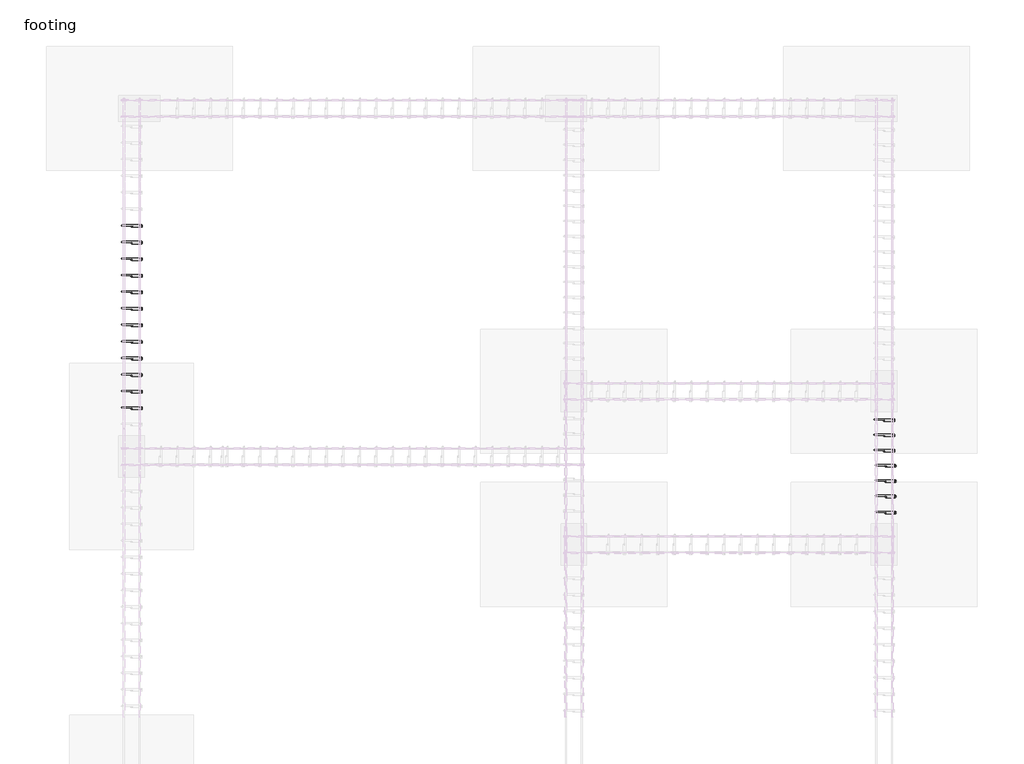
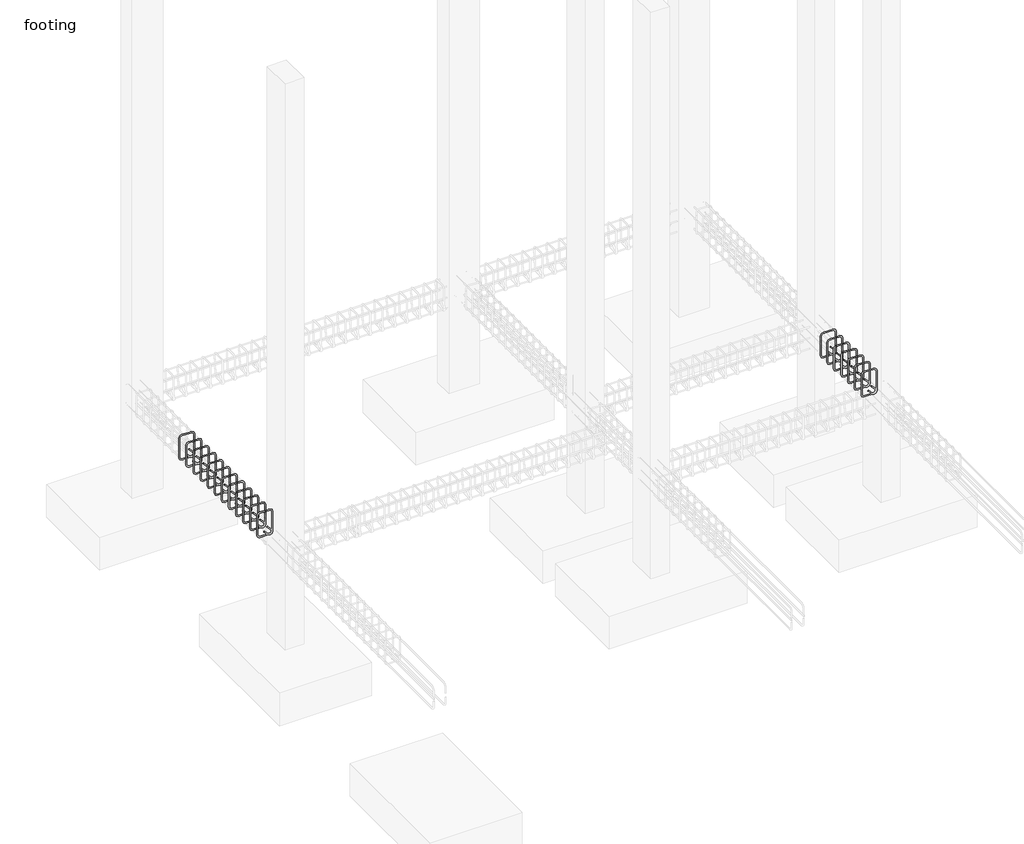
# One storey, part 15 of 21: 19 reinforcing bars.
"""IFC4 building model written with IfcOpenShell, lengths in millimetres."""

from ifc_helpers import new_model, si_unit, point, frame, origin, place, context, project, spatial, polyline, circle_curve, trimmed, segment, composite_curve, element, save
from ifc_brep_helpers import swept_disk

model = new_model("IFC4")

# Units and contexts
model_context = context("Model", 3, world=origin())
ifc_project = project(units=[si_unit("LENGTHUNIT", "METRE", prefix="MILLI")], contexts=[model_context])

# Site, building, storey
site = spatial("IfcSite", under=ifc_project)
building = spatial("IfcBuilding", under=site)
storey = spatial("IfcBuildingStorey", under=building, Name="footing", Elevation=-1524.0)

# Reinforcing bars
placement = place(None, origin())
element("IfcReinforcingBar", 1, at=placement, inside=storey, context=model_context, shape_type="SolidModel", body=[
    swept_disk(composite_curve([segment(polyline([(-12178.1165254, 8042.8456073, -265.9812362), (-12123.251527, 8042.8456073, -320.8462347)]), True, "CONTINUOUS"), segment(trimmed(circle_curve(frame((-12145.7021673, 8042.8456073, -343.296875), z_axis=(0.0, 1.0, 0.0), x_axis=(22.450640299999577, 0.0, 22.450640299999975)), 31.75), [point((-12123.251527, 8042.8456073, -320.8462347))], [point((-12145.7021673, 8042.8456073, -375.046875))], True, "CARTESIAN"), True, "CONTINUOUS"), segment(polyline([(-12145.7021673, 8042.8456073, -375.046875), (-12273.4959173, 8042.8456073, -375.046875)]), True, "CONTINUOUS"), segment(trimmed(circle_curve(frame((-12273.4959173, 8042.8456073, -343.296875), z_axis=(0.0, 1.0, 0.0), x_axis=(0.0, 0.0, -31.75)), 31.75), [point((-12273.4959173, 8042.8456073, -375.046875))], [point((-12305.2459173, 8042.8456073, -343.296875))], True, "CARTESIAN"), True, "CONTINUOUS"), segment(polyline([(-12305.2459173, 8042.8456073, -343.296875), (-12305.2459173, 8042.8456073, -63.103125)]), True, "CONTINUOUS"), segment(trimmed(circle_curve(frame((-12273.565658, 8040.7423536, -63.103125), z_axis=(0.0662442117686417, 0.9978034397651431, 0.0), x_axis=(-31.680259300001126, 2.1032537000000957, 0.0)), 31.75), [point((-12305.2459173, 8042.8456073, -63.103125))], [point((-12273.565658, 8040.7423536, -31.353125))], True, "CARTESIAN"), True, "CONTINUOUS"), segment(polyline([(-12273.565658, 8040.7423536, -31.353125), (-12145.6324265, 8032.248861, -31.353125)]), True, "CONTINUOUS"), segment(trimmed(circle_curve(frame((-12145.6324265, 8032.248861, -63.103125), z_axis=(0.06624421176864169, 0.997803439765143, 0.0), x_axis=(0.0, 0.0, 31.75)), 31.75), [point((-12145.6324265, 8032.248861, -31.353125))], [point((-12113.9521673, 8030.1456073, -63.103125))], True, "CARTESIAN"), True, "CONTINUOUS"), segment(polyline([(-12113.9521673, 8030.1456073, -63.103125), (-12113.9521673, 8030.1456073, -343.296875)]), True, "CONTINUOUS"), segment(trimmed(circle_curve(frame((-12145.7021673, 8030.1456073, -343.296875), z_axis=(0.0, 1.0, 0.0), x_axis=(31.75, 0.0, 0.0)), 31.75), [point((-12113.9521673, 8030.1456073, -343.296875))], [point((-12168.1528076, 8030.1456073, -365.7475153))], True, "CARTESIAN"), True, "CONTINUOUS"), segment(polyline([(-12168.1528076, 8030.1456073, -365.7475153), (-12223.017806, 8030.1456073, -310.8825168)]), True, "CONTINUOUS")], self_intersect=False), 6.35),
])
element("IfcReinforcingBar", 2, at=placement, inside=storey, context=model_context, shape_type="SolidModel", body=[
    swept_disk(composite_curve([segment(polyline([(-12178.1165254, 8205.5456073, -265.9812362), (-12123.251527, 8205.5456073, -320.8462347)]), True, "CONTINUOUS"), segment(trimmed(circle_curve(frame((-12145.7021673, 8205.5456073, -343.296875), z_axis=(0.0, 1.0, 0.0), x_axis=(22.450640299999577, 0.0, 22.450640299999975)), 31.75), [point((-12123.251527, 8205.5456073, -320.8462347))], [point((-12145.7021673, 8205.5456073, -375.046875))], True, "CARTESIAN"), True, "CONTINUOUS"), segment(polyline([(-12145.7021673, 8205.5456073, -375.046875), (-12273.4959173, 8205.5456073, -375.046875)]), True, "CONTINUOUS"), segment(trimmed(circle_curve(frame((-12273.4959173, 8205.5456073, -343.296875), z_axis=(0.0, 1.0, 0.0), x_axis=(0.0, 0.0, -31.75)), 31.75), [point((-12273.4959173, 8205.5456073, -375.046875))], [point((-12305.2459173, 8205.5456073, -343.296875))], True, "CARTESIAN"), True, "CONTINUOUS"), segment(polyline([(-12305.2459173, 8205.5456073, -343.296875), (-12305.2459173, 8205.5456073, -63.103125)]), True, "CONTINUOUS"), segment(trimmed(circle_curve(frame((-12273.565658, 8203.4423536, -63.103125), z_axis=(0.0662442117686417, 0.9978034397651431, 0.0), x_axis=(-31.680259300001126, 2.103253700001005, 0.0)), 31.75), [point((-12305.2459173, 8205.5456073, -63.103125))], [point((-12273.565658, 8203.4423536, -31.353125))], True, "CARTESIAN"), True, "CONTINUOUS"), segment(polyline([(-12273.565658, 8203.4423536, -31.353125), (-12145.6324265, 8194.948861, -31.353125)]), True, "CONTINUOUS"), segment(trimmed(circle_curve(frame((-12145.6324265, 8194.948861, -63.103125), z_axis=(0.06624421176864169, 0.997803439765143, 0.0), x_axis=(0.0, 0.0, 31.75)), 31.75), [point((-12145.6324265, 8194.948861, -31.353125))], [point((-12113.9521673, 8192.8456073, -63.103125))], True, "CARTESIAN"), True, "CONTINUOUS"), segment(polyline([(-12113.9521673, 8192.8456073, -63.103125), (-12113.9521673, 8192.8456073, -343.296875)]), True, "CONTINUOUS"), segment(trimmed(circle_curve(frame((-12145.7021673, 8192.8456073, -343.296875), z_axis=(0.0, 1.0, 0.0), x_axis=(31.75, 0.0, 0.0)), 31.75), [point((-12113.9521673, 8192.8456073, -343.296875))], [point((-12168.1528076, 8192.8456073, -365.7475153))], True, "CARTESIAN"), True, "CONTINUOUS"), segment(polyline([(-12168.1528076, 8192.8456073, -365.7475153), (-12223.017806, 8192.8456073, -310.8825168)]), True, "CONTINUOUS")], self_intersect=False), 6.35),
])
element("IfcReinforcingBar", 3, at=placement, inside=storey, context=model_context, shape_type="SolidModel", body=[
    swept_disk(composite_curve([segment(polyline([(-12178.1165254, 8368.2456073, -265.9812362), (-12123.251527, 8368.2456073, -320.8462347)]), True, "CONTINUOUS"), segment(trimmed(circle_curve(frame((-12145.7021673, 8368.2456073, -343.296875), z_axis=(0.0, 1.0, 0.0), x_axis=(22.450640299999577, 0.0, 22.450640299999975)), 31.75), [point((-12123.251527, 8368.2456073, -320.8462347))], [point((-12145.7021673, 8368.2456073, -375.046875))], True, "CARTESIAN"), True, "CONTINUOUS"), segment(polyline([(-12145.7021673, 8368.2456073, -375.046875), (-12273.4959173, 8368.2456073, -375.046875)]), True, "CONTINUOUS"), segment(trimmed(circle_curve(frame((-12273.4959173, 8368.2456073, -343.296875), z_axis=(0.0, 1.0, 0.0), x_axis=(0.0, 0.0, -31.75)), 31.75), [point((-12273.4959173, 8368.2456073, -375.046875))], [point((-12305.2459173, 8368.2456073, -343.296875))], True, "CARTESIAN"), True, "CONTINUOUS"), segment(polyline([(-12305.2459173, 8368.2456073, -343.296875), (-12305.2459173, 8368.2456073, -63.103125)]), True, "CONTINUOUS"), segment(trimmed(circle_curve(frame((-12273.565658, 8366.1423536, -63.103125), z_axis=(0.0662442117686417, 0.9978034397651431, 0.0), x_axis=(-31.680259300001126, 2.103253699999186, 0.0)), 31.75), [point((-12305.2459173, 8368.2456073, -63.103125))], [point((-12273.565658, 8366.1423536, -31.353125))], True, "CARTESIAN"), True, "CONTINUOUS"), segment(polyline([(-12273.565658, 8366.1423536, -31.353125), (-12145.6324265, 8357.648861, -31.353125)]), True, "CONTINUOUS"), segment(trimmed(circle_curve(frame((-12145.6324265, 8357.648861, -63.103125), z_axis=(0.06624421176864169, 0.997803439765143, 0.0), x_axis=(0.0, 0.0, 31.75)), 31.75), [point((-12145.6324265, 8357.648861, -31.353125))], [point((-12113.9521673, 8355.5456073, -63.103125))], True, "CARTESIAN"), True, "CONTINUOUS"), segment(polyline([(-12113.9521673, 8355.5456073, -63.103125), (-12113.9521673, 8355.5456073, -343.296875)]), True, "CONTINUOUS"), segment(trimmed(circle_curve(frame((-12145.7021673, 8355.5456073, -343.296875), z_axis=(0.0, 1.0, 0.0), x_axis=(31.75, 0.0, 0.0)), 31.75), [point((-12113.9521673, 8355.5456073, -343.296875))], [point((-12168.1528076, 8355.5456073, -365.7475153))], True, "CARTESIAN"), True, "CONTINUOUS"), segment(polyline([(-12168.1528076, 8355.5456073, -365.7475153), (-12223.017806, 8355.5456073, -310.8825168)]), True, "CONTINUOUS")], self_intersect=False), 6.35),
])
element("IfcReinforcingBar", 4, at=placement, inside=storey, context=model_context, shape_type="SolidModel", body=[
    swept_disk(composite_curve([segment(polyline([(-12178.1165254, 8530.9456073, -265.9812362), (-12123.251527, 8530.9456073, -320.8462347)]), True, "CONTINUOUS"), segment(trimmed(circle_curve(frame((-12145.7021673, 8530.9456073, -343.296875), z_axis=(0.0, 1.0, 0.0), x_axis=(22.450640299999577, 0.0, 22.450640299999975)), 31.75), [point((-12123.251527, 8530.9456073, -320.8462347))], [point((-12145.7021673, 8530.9456073, -375.046875))], True, "CARTESIAN"), True, "CONTINUOUS"), segment(polyline([(-12145.7021673, 8530.9456073, -375.046875), (-12273.4959173, 8530.9456073, -375.046875)]), True, "CONTINUOUS"), segment(trimmed(circle_curve(frame((-12273.4959173, 8530.9456073, -343.296875), z_axis=(0.0, 1.0, 0.0), x_axis=(0.0, 0.0, -31.75)), 31.75), [point((-12273.4959173, 8530.9456073, -375.046875))], [point((-12305.2459173, 8530.9456073, -343.296875))], True, "CARTESIAN"), True, "CONTINUOUS"), segment(polyline([(-12305.2459173, 8530.9456073, -343.296875), (-12305.2459173, 8530.9456073, -63.103125)]), True, "CONTINUOUS"), segment(trimmed(circle_curve(frame((-12273.565658, 8528.8423536, -63.103125), z_axis=(0.0662442117686417, 0.9978034397651431, 0.0), x_axis=(-31.680259300001126, 2.103253700001005, 0.0)), 31.75), [point((-12305.2459173, 8530.9456073, -63.103125))], [point((-12273.565658, 8528.8423536, -31.353125))], True, "CARTESIAN"), True, "CONTINUOUS"), segment(polyline([(-12273.565658, 8528.8423536, -31.353125), (-12145.6324265, 8520.348861, -31.353125)]), True, "CONTINUOUS"), segment(trimmed(circle_curve(frame((-12145.6324265, 8520.348861, -63.103125), z_axis=(0.06624421176864169, 0.997803439765143, 0.0), x_axis=(0.0, 0.0, 31.75)), 31.75), [point((-12145.6324265, 8520.348861, -31.353125))], [point((-12113.9521673, 8518.2456073, -63.103125))], True, "CARTESIAN"), True, "CONTINUOUS"), segment(polyline([(-12113.9521673, 8518.2456073, -63.103125), (-12113.9521673, 8518.2456073, -343.296875)]), True, "CONTINUOUS"), segment(trimmed(circle_curve(frame((-12145.7021673, 8518.2456073, -343.296875), z_axis=(0.0, 1.0, 0.0), x_axis=(31.75, 0.0, 0.0)), 31.75), [point((-12113.9521673, 8518.2456073, -343.296875))], [point((-12168.1528076, 8518.2456073, -365.7475153))], True, "CARTESIAN"), True, "CONTINUOUS"), segment(polyline([(-12168.1528076, 8518.2456073, -365.7475153), (-12223.017806, 8518.2456073, -310.8825168)]), True, "CONTINUOUS")], self_intersect=False), 6.35),
])
element("IfcReinforcingBar", 5, at=placement, inside=storey, context=model_context, shape_type="SolidModel", body=[
    swept_disk(composite_curve([segment(polyline([(-12178.1165254, 8693.6456073, -265.9812362), (-12123.251527, 8693.6456073, -320.8462347)]), True, "CONTINUOUS"), segment(trimmed(circle_curve(frame((-12145.7021673, 8693.6456073, -343.296875), z_axis=(0.0, 1.0, 0.0), x_axis=(22.450640299999577, 0.0, 22.450640299999975)), 31.75), [point((-12123.251527, 8693.6456073, -320.8462347))], [point((-12145.7021673, 8693.6456073, -375.046875))], True, "CARTESIAN"), True, "CONTINUOUS"), segment(polyline([(-12145.7021673, 8693.6456073, -375.046875), (-12273.4959173, 8693.6456073, -375.046875)]), True, "CONTINUOUS"), segment(trimmed(circle_curve(frame((-12273.4959173, 8693.6456073, -343.296875), z_axis=(0.0, 1.0, 0.0), x_axis=(0.0, 0.0, -31.75)), 31.75), [point((-12273.4959173, 8693.6456073, -375.046875))], [point((-12305.2459173, 8693.6456073, -343.296875))], True, "CARTESIAN"), True, "CONTINUOUS"), segment(polyline([(-12305.2459173, 8693.6456073, -343.296875), (-12305.2459173, 8693.6456073, -63.103125)]), True, "CONTINUOUS"), segment(trimmed(circle_curve(frame((-12273.565658, 8691.5423536, -63.103125), z_axis=(0.0662442117686417, 0.9978034397651431, 0.0), x_axis=(-31.680259300001126, 2.103253700001005, 0.0)), 31.75), [point((-12305.2459173, 8693.6456073, -63.103125))], [point((-12273.565658, 8691.5423536, -31.353125))], True, "CARTESIAN"), True, "CONTINUOUS"), segment(polyline([(-12273.565658, 8691.5423536, -31.353125), (-12145.6324265, 8683.048861, -31.353125)]), True, "CONTINUOUS"), segment(trimmed(circle_curve(frame((-12145.6324265, 8683.048861, -63.103125), z_axis=(0.06624421176864169, 0.997803439765143, 0.0), x_axis=(0.0, 0.0, 31.75)), 31.75), [point((-12145.6324265, 8683.048861, -31.353125))], [point((-12113.9521673, 8680.9456073, -63.103125))], True, "CARTESIAN"), True, "CONTINUOUS"), segment(polyline([(-12113.9521673, 8680.9456073, -63.103125), (-12113.9521673, 8680.9456073, -343.296875)]), True, "CONTINUOUS"), segment(trimmed(circle_curve(frame((-12145.7021673, 8680.9456073, -343.296875), z_axis=(0.0, 1.0, 0.0), x_axis=(31.75, 0.0, 0.0)), 31.75), [point((-12113.9521673, 8680.9456073, -343.296875))], [point((-12168.1528076, 8680.9456073, -365.7475153))], True, "CARTESIAN"), True, "CONTINUOUS"), segment(polyline([(-12168.1528076, 8680.9456073, -365.7475153), (-12223.017806, 8680.9456073, -310.8825168)]), True, "CONTINUOUS")], self_intersect=False), 6.35),
])
element("IfcReinforcingBar", 6, at=placement, inside=storey, context=model_context, shape_type="SolidModel", body=[
    swept_disk(composite_curve([segment(polyline([(-12178.1165254, 8856.3456073, -265.9812362), (-12123.251527, 8856.3456073, -320.8462347)]), True, "CONTINUOUS"), segment(trimmed(circle_curve(frame((-12145.7021673, 8856.3456073, -343.296875), z_axis=(0.0, 1.0, 0.0), x_axis=(22.450640299999577, 0.0, 22.450640299999975)), 31.75), [point((-12123.251527, 8856.3456073, -320.8462347))], [point((-12145.7021673, 8856.3456073, -375.046875))], True, "CARTESIAN"), True, "CONTINUOUS"), segment(polyline([(-12145.7021673, 8856.3456073, -375.046875), (-12273.4959173, 8856.3456073, -375.046875)]), True, "CONTINUOUS"), segment(trimmed(circle_curve(frame((-12273.4959173, 8856.3456073, -343.296875), z_axis=(0.0, 1.0, 0.0), x_axis=(0.0, 0.0, -31.75)), 31.75), [point((-12273.4959173, 8856.3456073, -375.046875))], [point((-12305.2459173, 8856.3456073, -343.296875))], True, "CARTESIAN"), True, "CONTINUOUS"), segment(polyline([(-12305.2459173, 8856.3456073, -343.296875), (-12305.2459173, 8856.3456073, -63.103125)]), True, "CONTINUOUS"), segment(trimmed(circle_curve(frame((-12273.565658, 8854.2423536, -63.103125), z_axis=(0.0662442117686417, 0.9978034397651431, 0.0), x_axis=(-31.680259300001126, 2.103253699999186, 0.0)), 31.75), [point((-12305.2459173, 8856.3456073, -63.103125))], [point((-12273.565658, 8854.2423536, -31.353125))], True, "CARTESIAN"), True, "CONTINUOUS"), segment(polyline([(-12273.565658, 8854.2423536, -31.353125), (-12145.6324265, 8845.748861, -31.353125)]), True, "CONTINUOUS"), segment(trimmed(circle_curve(frame((-12145.6324265, 8845.748861, -63.103125), z_axis=(0.06624421176864169, 0.997803439765143, 0.0), x_axis=(0.0, 0.0, 31.75)), 31.75), [point((-12145.6324265, 8845.748861, -31.353125))], [point((-12113.9521673, 8843.6456073, -63.103125))], True, "CARTESIAN"), True, "CONTINUOUS"), segment(polyline([(-12113.9521673, 8843.6456073, -63.103125), (-12113.9521673, 8843.6456073, -343.296875)]), True, "CONTINUOUS"), segment(trimmed(circle_curve(frame((-12145.7021673, 8843.6456073, -343.296875), z_axis=(0.0, 1.0, 0.0), x_axis=(31.75, 0.0, 0.0)), 31.75), [point((-12113.9521673, 8843.6456073, -343.296875))], [point((-12168.1528076, 8843.6456073, -365.7475153))], True, "CARTESIAN"), True, "CONTINUOUS"), segment(polyline([(-12168.1528076, 8843.6456073, -365.7475153), (-12223.017806, 8843.6456073, -310.8825168)]), True, "CONTINUOUS")], self_intersect=False), 6.35),
])
element("IfcReinforcingBar", 7, at=placement, inside=storey, context=model_context, shape_type="SolidModel", body=[
    swept_disk(composite_curve([segment(polyline([(-12178.1165254, 9019.0456073, -265.9812362), (-12123.251527, 9019.0456073, -320.8462347)]), True, "CONTINUOUS"), segment(trimmed(circle_curve(frame((-12145.7021673, 9019.0456073, -343.296875), z_axis=(0.0, 1.0, 0.0), x_axis=(22.450640299999577, 0.0, 22.450640299999975)), 31.75), [point((-12123.251527, 9019.0456073, -320.8462347))], [point((-12145.7021673, 9019.0456073, -375.046875))], True, "CARTESIAN"), True, "CONTINUOUS"), segment(polyline([(-12145.7021673, 9019.0456073, -375.046875), (-12273.4959173, 9019.0456073, -375.046875)]), True, "CONTINUOUS"), segment(trimmed(circle_curve(frame((-12273.4959173, 9019.0456073, -343.296875), z_axis=(0.0, 1.0, 0.0), x_axis=(0.0, 0.0, -31.75)), 31.75), [point((-12273.4959173, 9019.0456073, -375.046875))], [point((-12305.2459173, 9019.0456073, -343.296875))], True, "CARTESIAN"), True, "CONTINUOUS"), segment(polyline([(-12305.2459173, 9019.0456073, -343.296875), (-12305.2459173, 9019.0456073, -63.103125)]), True, "CONTINUOUS"), segment(trimmed(circle_curve(frame((-12273.565658, 9016.9423536, -63.103125), z_axis=(0.0662442117686417, 0.9978034397651431, 0.0), x_axis=(-31.680259300001126, 2.103253700001005, 0.0)), 31.75), [point((-12305.2459173, 9019.0456073, -63.103125))], [point((-12273.565658, 9016.9423536, -31.353125))], True, "CARTESIAN"), True, "CONTINUOUS"), segment(polyline([(-12273.565658, 9016.9423536, -31.353125), (-12145.6324265, 9008.448861, -31.353125)]), True, "CONTINUOUS"), segment(trimmed(circle_curve(frame((-12145.6324265, 9008.448861, -63.103125), z_axis=(0.06624421176864169, 0.997803439765143, 0.0), x_axis=(0.0, 0.0, 31.75)), 31.75), [point((-12145.6324265, 9008.448861, -31.353125))], [point((-12113.9521673, 9006.3456073, -63.103125))], True, "CARTESIAN"), True, "CONTINUOUS"), segment(polyline([(-12113.9521673, 9006.3456073, -63.103125), (-12113.9521673, 9006.3456073, -343.296875)]), True, "CONTINUOUS"), segment(trimmed(circle_curve(frame((-12145.7021673, 9006.3456073, -343.296875), z_axis=(0.0, 1.0, 0.0), x_axis=(31.75, 0.0, 0.0)), 31.75), [point((-12113.9521673, 9006.3456073, -343.296875))], [point((-12168.1528076, 9006.3456073, -365.7475153))], True, "CARTESIAN"), True, "CONTINUOUS"), segment(polyline([(-12168.1528076, 9006.3456073, -365.7475153), (-12223.017806, 9006.3456073, -310.8825168)]), True, "CONTINUOUS")], self_intersect=False), 6.35),
])
element("IfcReinforcingBar", 8, at=placement, inside=storey, context=model_context, shape_type="SolidModel", body=[
    swept_disk(composite_curve([segment(polyline([(-12178.1165254, 9181.7456073, -265.9812362), (-12123.251527, 9181.7456073, -320.8462347)]), True, "CONTINUOUS"), segment(trimmed(circle_curve(frame((-12145.7021673, 9181.7456073, -343.296875), z_axis=(0.0, 1.0, 0.0), x_axis=(22.450640299999577, 0.0, 22.450640299999975)), 31.75), [point((-12123.251527, 9181.7456073, -320.8462347))], [point((-12145.7021673, 9181.7456073, -375.046875))], True, "CARTESIAN"), True, "CONTINUOUS"), segment(polyline([(-12145.7021673, 9181.7456073, -375.046875), (-12273.4959173, 9181.7456073, -375.046875)]), True, "CONTINUOUS"), segment(trimmed(circle_curve(frame((-12273.4959173, 9181.7456073, -343.296875), z_axis=(0.0, 1.0, 0.0), x_axis=(0.0, 0.0, -31.75)), 31.75), [point((-12273.4959173, 9181.7456073, -375.046875))], [point((-12305.2459173, 9181.7456073, -343.296875))], True, "CARTESIAN"), True, "CONTINUOUS"), segment(polyline([(-12305.2459173, 9181.7456073, -343.296875), (-12305.2459173, 9181.7456073, -63.103125)]), True, "CONTINUOUS"), segment(trimmed(circle_curve(frame((-12273.565658, 9179.6423536, -63.103125), z_axis=(0.0662442117686417, 0.9978034397651431, 0.0), x_axis=(-31.680259300001126, 2.103253699999186, 0.0)), 31.75), [point((-12305.2459173, 9181.7456073, -63.103125))], [point((-12273.565658, 9179.6423536, -31.353125))], True, "CARTESIAN"), True, "CONTINUOUS"), segment(polyline([(-12273.565658, 9179.6423536, -31.353125), (-12145.6324265, 9171.148861, -31.353125)]), True, "CONTINUOUS"), segment(trimmed(circle_curve(frame((-12145.6324265, 9171.148861, -63.103125), z_axis=(0.06624421176864169, 0.997803439765143, 0.0), x_axis=(0.0, 0.0, 31.75)), 31.75), [point((-12145.6324265, 9171.148861, -31.353125))], [point((-12113.9521673, 9169.0456073, -63.103125))], True, "CARTESIAN"), True, "CONTINUOUS"), segment(polyline([(-12113.9521673, 9169.0456073, -63.103125), (-12113.9521673, 9169.0456073, -343.296875)]), True, "CONTINUOUS"), segment(trimmed(circle_curve(frame((-12145.7021673, 9169.0456073, -343.296875), z_axis=(0.0, 1.0, 0.0), x_axis=(31.75, 0.0, 0.0)), 31.75), [point((-12113.9521673, 9169.0456073, -343.296875))], [point((-12168.1528076, 9169.0456073, -365.7475153))], True, "CARTESIAN"), True, "CONTINUOUS"), segment(polyline([(-12168.1528076, 9169.0456073, -365.7475153), (-12223.017806, 9169.0456073, -310.8825168)]), True, "CONTINUOUS")], self_intersect=False), 6.35),
])
element("IfcReinforcingBar", 9, at=placement, inside=storey, context=model_context, shape_type="SolidModel", body=[
    swept_disk(composite_curve([segment(polyline([(-12178.1165254, 9344.4456073, -265.9812362), (-12123.251527, 9344.4456073, -320.8462347)]), True, "CONTINUOUS"), segment(trimmed(circle_curve(frame((-12145.7021673, 9344.4456073, -343.296875), z_axis=(0.0, 1.0, 0.0), x_axis=(22.450640299999577, 0.0, 22.450640299999975)), 31.75), [point((-12123.251527, 9344.4456073, -320.8462347))], [point((-12145.7021673, 9344.4456073, -375.046875))], True, "CARTESIAN"), True, "CONTINUOUS"), segment(polyline([(-12145.7021673, 9344.4456073, -375.046875), (-12273.4959173, 9344.4456073, -375.046875)]), True, "CONTINUOUS"), segment(trimmed(circle_curve(frame((-12273.4959173, 9344.4456073, -343.296875), z_axis=(0.0, 1.0, 0.0), x_axis=(0.0, 0.0, -31.75)), 31.75), [point((-12273.4959173, 9344.4456073, -375.046875))], [point((-12305.2459173, 9344.4456073, -343.296875))], True, "CARTESIAN"), True, "CONTINUOUS"), segment(polyline([(-12305.2459173, 9344.4456073, -343.296875), (-12305.2459173, 9344.4456073, -63.103125)]), True, "CONTINUOUS"), segment(trimmed(circle_curve(frame((-12273.565658, 9342.3423536, -63.103125), z_axis=(0.0662442117686417, 0.9978034397651431, 0.0), x_axis=(-31.680259300001126, 2.103253700001005, 0.0)), 31.75), [point((-12305.2459173, 9344.4456073, -63.103125))], [point((-12273.565658, 9342.3423536, -31.353125))], True, "CARTESIAN"), True, "CONTINUOUS"), segment(polyline([(-12273.565658, 9342.3423536, -31.353125), (-12145.6324265, 9333.848861, -31.353125)]), True, "CONTINUOUS"), segment(trimmed(circle_curve(frame((-12145.6324265, 9333.848861, -63.103125), z_axis=(0.06624421176864169, 0.997803439765143, 0.0), x_axis=(0.0, 0.0, 31.75)), 31.75), [point((-12145.6324265, 9333.848861, -31.353125))], [point((-12113.9521673, 9331.7456073, -63.103125))], True, "CARTESIAN"), True, "CONTINUOUS"), segment(polyline([(-12113.9521673, 9331.7456073, -63.103125), (-12113.9521673, 9331.7456073, -343.296875)]), True, "CONTINUOUS"), segment(trimmed(circle_curve(frame((-12145.7021673, 9331.7456073, -343.296875), z_axis=(0.0, 1.0, 0.0), x_axis=(31.75, 0.0, 0.0)), 31.75), [point((-12113.9521673, 9331.7456073, -343.296875))], [point((-12168.1528076, 9331.7456073, -365.7475153))], True, "CARTESIAN"), True, "CONTINUOUS"), segment(polyline([(-12168.1528076, 9331.7456073, -365.7475153), (-12223.017806, 9331.7456073, -310.8825168)]), True, "CONTINUOUS")], self_intersect=False), 6.35),
])
element("IfcReinforcingBar", 10, at=placement, inside=storey, context=model_context, shape_type="SolidModel", body=[
    swept_disk(composite_curve([segment(polyline([(-12178.1165254, 9507.1456073, -265.9812362), (-12123.251527, 9507.1456073, -320.8462347)]), True, "CONTINUOUS"), segment(trimmed(circle_curve(frame((-12145.7021673, 9507.1456073, -343.296875), z_axis=(0.0, 1.0, 0.0), x_axis=(22.450640299999577, 0.0, 22.450640299999975)), 31.75), [point((-12123.251527, 9507.1456073, -320.8462347))], [point((-12145.7021673, 9507.1456073, -375.046875))], True, "CARTESIAN"), True, "CONTINUOUS"), segment(polyline([(-12145.7021673, 9507.1456073, -375.046875), (-12273.4959173, 9507.1456073, -375.046875)]), True, "CONTINUOUS"), segment(trimmed(circle_curve(frame((-12273.4959173, 9507.1456073, -343.296875), z_axis=(0.0, 1.0, 0.0), x_axis=(0.0, 0.0, -31.75)), 31.75), [point((-12273.4959173, 9507.1456073, -375.046875))], [point((-12305.2459173, 9507.1456073, -343.296875))], True, "CARTESIAN"), True, "CONTINUOUS"), segment(polyline([(-12305.2459173, 9507.1456073, -343.296875), (-12305.2459173, 9507.1456073, -63.103125)]), True, "CONTINUOUS"), segment(trimmed(circle_curve(frame((-12273.565658, 9505.0423536, -63.103125), z_axis=(0.0662442117686417, 0.9978034397651431, 0.0), x_axis=(-31.680259300001126, 2.103253700001005, 0.0)), 31.75), [point((-12305.2459173, 9507.1456073, -63.103125))], [point((-12273.565658, 9505.0423536, -31.353125))], True, "CARTESIAN"), True, "CONTINUOUS"), segment(polyline([(-12273.565658, 9505.0423536, -31.353125), (-12145.6324265, 9496.548861, -31.353125)]), True, "CONTINUOUS"), segment(trimmed(circle_curve(frame((-12145.6324265, 9496.548861, -63.103125), z_axis=(0.06624421176864169, 0.997803439765143, 0.0), x_axis=(0.0, 0.0, 31.75)), 31.75), [point((-12145.6324265, 9496.548861, -31.353125))], [point((-12113.9521673, 9494.4456073, -63.103125))], True, "CARTESIAN"), True, "CONTINUOUS"), segment(polyline([(-12113.9521673, 9494.4456073, -63.103125), (-12113.9521673, 9494.4456073, -343.296875)]), True, "CONTINUOUS"), segment(trimmed(circle_curve(frame((-12145.7021673, 9494.4456073, -343.296875), z_axis=(0.0, 1.0, 0.0), x_axis=(31.75, 0.0, 0.0)), 31.75), [point((-12113.9521673, 9494.4456073, -343.296875))], [point((-12168.1528076, 9494.4456073, -365.7475153))], True, "CARTESIAN"), True, "CONTINUOUS"), segment(polyline([(-12168.1528076, 9494.4456073, -365.7475153), (-12223.017806, 9494.4456073, -310.8825168)]), True, "CONTINUOUS")], self_intersect=False), 6.35),
])
element("IfcReinforcingBar", 11, at=placement, inside=storey, context=model_context, shape_type="SolidModel", body=[
    swept_disk(composite_curve([segment(polyline([(-12178.1165254, 9669.8456073, -265.9812362), (-12123.251527, 9669.8456073, -320.8462347)]), True, "CONTINUOUS"), segment(trimmed(circle_curve(frame((-12145.7021673, 9669.8456073, -343.296875), z_axis=(0.0, 1.0, 0.0), x_axis=(22.450640299999577, 0.0, 22.450640299999975)), 31.75), [point((-12123.251527, 9669.8456073, -320.8462347))], [point((-12145.7021673, 9669.8456073, -375.046875))], True, "CARTESIAN"), True, "CONTINUOUS"), segment(polyline([(-12145.7021673, 9669.8456073, -375.046875), (-12273.4959173, 9669.8456073, -375.046875)]), True, "CONTINUOUS"), segment(trimmed(circle_curve(frame((-12273.4959173, 9669.8456073, -343.296875), z_axis=(0.0, 1.0, 0.0), x_axis=(0.0, 0.0, -31.75)), 31.75), [point((-12273.4959173, 9669.8456073, -375.046875))], [point((-12305.2459173, 9669.8456073, -343.296875))], True, "CARTESIAN"), True, "CONTINUOUS"), segment(polyline([(-12305.2459173, 9669.8456073, -343.296875), (-12305.2459173, 9669.8456073, -63.103125)]), True, "CONTINUOUS"), segment(trimmed(circle_curve(frame((-12273.565658, 9667.7423536, -63.103125), z_axis=(0.0662442117686417, 0.9978034397651431, 0.0), x_axis=(-31.680259300001126, 2.103253699999186, 0.0)), 31.75), [point((-12305.2459173, 9669.8456073, -63.103125))], [point((-12273.565658, 9667.7423536, -31.353125))], True, "CARTESIAN"), True, "CONTINUOUS"), segment(polyline([(-12273.565658, 9667.7423536, -31.353125), (-12145.6324265, 9659.248861, -31.353125)]), True, "CONTINUOUS"), segment(trimmed(circle_curve(frame((-12145.6324265, 9659.248861, -63.103125), z_axis=(0.06624421176864169, 0.997803439765143, 0.0), x_axis=(0.0, 0.0, 31.75)), 31.75), [point((-12145.6324265, 9659.248861, -31.353125))], [point((-12113.9521673, 9657.1456073, -63.103125))], True, "CARTESIAN"), True, "CONTINUOUS"), segment(polyline([(-12113.9521673, 9657.1456073, -63.103125), (-12113.9521673, 9657.1456073, -343.296875)]), True, "CONTINUOUS"), segment(trimmed(circle_curve(frame((-12145.7021673, 9657.1456073, -343.296875), z_axis=(0.0, 1.0, 0.0), x_axis=(31.75, 0.0, 0.0)), 31.75), [point((-12113.9521673, 9657.1456073, -343.296875))], [point((-12168.1528076, 9657.1456073, -365.7475153))], True, "CARTESIAN"), True, "CONTINUOUS"), segment(polyline([(-12168.1528076, 9657.1456073, -365.7475153), (-12223.017806, 9657.1456073, -310.8825168)]), True, "CONTINUOUS")], self_intersect=False), 6.35),
])
element("IfcReinforcingBar", 12, at=placement, inside=storey, context=model_context, shape_type="SolidModel", body=[
    swept_disk(composite_curve([segment(polyline([(-12178.1165254, 9832.5456073, -265.9812362), (-12123.251527, 9832.5456073, -320.8462347)]), True, "CONTINUOUS"), segment(trimmed(circle_curve(frame((-12145.7021673, 9832.5456073, -343.296875), z_axis=(0.0, 1.0, 0.0), x_axis=(22.450640299999577, 0.0, 22.450640299999975)), 31.75), [point((-12123.251527, 9832.5456073, -320.8462347))], [point((-12145.7021673, 9832.5456073, -375.046875))], True, "CARTESIAN"), True, "CONTINUOUS"), segment(polyline([(-12145.7021673, 9832.5456073, -375.046875), (-12273.4959173, 9832.5456073, -375.046875)]), True, "CONTINUOUS"), segment(trimmed(circle_curve(frame((-12273.4959173, 9832.5456073, -343.296875), z_axis=(0.0, 1.0, 0.0), x_axis=(0.0, 0.0, -31.75)), 31.75), [point((-12273.4959173, 9832.5456073, -375.046875))], [point((-12305.2459173, 9832.5456073, -343.296875))], True, "CARTESIAN"), True, "CONTINUOUS"), segment(polyline([(-12305.2459173, 9832.5456073, -343.296875), (-12305.2459173, 9832.5456073, -63.103125)]), True, "CONTINUOUS"), segment(trimmed(circle_curve(frame((-12273.565658, 9830.4423536, -63.103125), z_axis=(0.0662442117686417, 0.9978034397651431, 0.0), x_axis=(-31.680259300001126, 2.103253700001005, 0.0)), 31.75), [point((-12305.2459173, 9832.5456073, -63.103125))], [point((-12273.565658, 9830.4423536, -31.353125))], True, "CARTESIAN"), True, "CONTINUOUS"), segment(polyline([(-12273.565658, 9830.4423536, -31.353125), (-12145.6324265, 9821.948861, -31.353125)]), True, "CONTINUOUS"), segment(trimmed(circle_curve(frame((-12145.6324265, 9821.948861, -63.103125), z_axis=(0.06624421176864169, 0.997803439765143, 0.0), x_axis=(0.0, 0.0, 31.75)), 31.75), [point((-12145.6324265, 9821.948861, -31.353125))], [point((-12113.9521673, 9819.8456073, -63.103125))], True, "CARTESIAN"), True, "CONTINUOUS"), segment(polyline([(-12113.9521673, 9819.8456073, -63.103125), (-12113.9521673, 9819.8456073, -343.296875)]), True, "CONTINUOUS"), segment(trimmed(circle_curve(frame((-12145.7021673, 9819.8456073, -343.296875), z_axis=(0.0, 1.0, 0.0), x_axis=(31.75, 0.0, 0.0)), 31.75), [point((-12113.9521673, 9819.8456073, -343.296875))], [point((-12168.1528076, 9819.8456073, -365.7475153))], True, "CARTESIAN"), True, "CONTINUOUS"), segment(polyline([(-12168.1528076, 9819.8456073, -365.7475153), (-12223.017806, 9819.8456073, -310.8825168)]), True, "CONTINUOUS")], self_intersect=False), 6.35),
])
element("IfcReinforcingBar", 13, at=placement, inside=storey, context=model_context, shape_type="SolidModel", body=[
    swept_disk(composite_curve([segment(polyline([(-4786.7165254, 7925.2699494, -265.9812362), (-4731.851527, 7925.2699494, -320.8462347)]), True, "CONTINUOUS"), segment(trimmed(circle_curve(frame((-4754.3021673, 7925.2699494, -343.296875), z_axis=(0.0, 1.0, 0.0), x_axis=(22.450640300000487, 0.0, 22.450640299999975)), 31.75), [point((-4731.851527, 7925.2699494, -320.8462347))], [point((-4754.3021673, 7925.2699494, -375.046875))], True, "CARTESIAN"), True, "CONTINUOUS"), segment(polyline([(-4754.3021673, 7925.2699494, -375.046875), (-4882.0959173, 7925.2699494, -375.046875)]), True, "CONTINUOUS"), segment(trimmed(circle_curve(frame((-4882.0959173, 7925.2699494, -343.296875), z_axis=(0.0, 1.0, 0.0), x_axis=(0.0, 0.0, -31.75)), 31.75), [point((-4882.0959173, 7925.2699494, -375.046875))], [point((-4913.8459173, 7925.2699494, -343.296875))], True, "CARTESIAN"), True, "CONTINUOUS"), segment(polyline([(-4913.8459173, 7925.2699494, -343.296875), (-4913.8459173, 7925.2699494, -63.103125)]), True, "CONTINUOUS"), segment(trimmed(circle_curve(frame((-4882.165658, 7923.1666957, -63.103125), z_axis=(0.06624421176864137, 0.9978034397651431, 0.0), x_axis=(-31.680259300000216, 2.1032537000000957, 0.0)), 31.75), [point((-4913.8459173, 7925.2699494, -63.103125))], [point((-4882.165658, 7923.1666957, -31.353125))], True, "CARTESIAN"), True, "CONTINUOUS"), segment(polyline([(-4882.165658, 7923.1666957, -31.353125), (-4754.2324265, 7914.6732031, -31.353125)]), True, "CONTINUOUS"), segment(trimmed(circle_curve(frame((-4754.2324265, 7914.6732031, -63.103125), z_axis=(0.06624421176864137, 0.9978034397651431, 0.0), x_axis=(0.0, 0.0, 31.75)), 31.75), [point((-4754.2324265, 7914.6732031, -31.353125))], [point((-4722.5521673, 7912.5699494, -63.103125))], True, "CARTESIAN"), True, "CONTINUOUS"), segment(polyline([(-4722.5521673, 7912.5699494, -63.103125), (-4722.5521673, 7912.5699494, -343.296875)]), True, "CONTINUOUS"), segment(trimmed(circle_curve(frame((-4754.3021673, 7912.5699494, -343.296875), z_axis=(0.0, 1.0, 0.0), x_axis=(31.75, 0.0, 0.0)), 31.75), [point((-4722.5521673, 7912.5699494, -343.296875))], [point((-4776.7528076, 7912.5699494, -365.7475153))], True, "CARTESIAN"), True, "CONTINUOUS"), segment(polyline([(-4776.7528076, 7912.5699494, -365.7475153), (-4831.617806, 7912.5699494, -310.8825168)]), True, "CONTINUOUS")], self_intersect=False), 6.35),
])
element("IfcReinforcingBar", 14, at=placement, inside=storey, context=model_context, shape_type="SolidModel", body=[
    swept_disk(composite_curve([segment(polyline([(-4786.7165254, 7775.2699494, -265.9812362), (-4731.851527, 7775.2699494, -320.8462347)]), True, "CONTINUOUS"), segment(trimmed(circle_curve(frame((-4754.3021673, 7775.2699494, -343.296875), z_axis=(0.0, 1.0, 0.0), x_axis=(22.450640300000487, 0.0, 22.450640299999975)), 31.75), [point((-4731.851527, 7775.2699494, -320.8462347))], [point((-4754.3021673, 7775.2699494, -375.046875))], True, "CARTESIAN"), True, "CONTINUOUS"), segment(polyline([(-4754.3021673, 7775.2699494, -375.046875), (-4882.0959173, 7775.2699494, -375.046875)]), True, "CONTINUOUS"), segment(trimmed(circle_curve(frame((-4882.0959173, 7775.2699494, -343.296875), z_axis=(0.0, 1.0, 0.0), x_axis=(0.0, 0.0, -31.75)), 31.75), [point((-4882.0959173, 7775.2699494, -375.046875))], [point((-4913.8459173, 7775.2699494, -343.296875))], True, "CARTESIAN"), True, "CONTINUOUS"), segment(polyline([(-4913.8459173, 7775.2699494, -343.296875), (-4913.8459173, 7775.2699494, -63.103125)]), True, "CONTINUOUS"), segment(trimmed(circle_curve(frame((-4882.165658, 7773.1666957, -63.103125), z_axis=(0.06624421176864137, 0.9978034397651431, 0.0), x_axis=(-31.680259300000216, 2.1032537000000957, 0.0)), 31.75), [point((-4913.8459173, 7775.2699494, -63.103125))], [point((-4882.165658, 7773.1666957, -31.353125))], True, "CARTESIAN"), True, "CONTINUOUS"), segment(polyline([(-4882.165658, 7773.1666957, -31.353125), (-4754.2324265, 7764.6732031, -31.353125)]), True, "CONTINUOUS"), segment(trimmed(circle_curve(frame((-4754.2324265, 7764.6732031, -63.103125), z_axis=(0.06624421176864137, 0.9978034397651431, 0.0), x_axis=(0.0, 0.0, 31.75)), 31.75), [point((-4754.2324265, 7764.6732031, -31.353125))], [point((-4722.5521673, 7762.5699494, -63.103125))], True, "CARTESIAN"), True, "CONTINUOUS"), segment(polyline([(-4722.5521673, 7762.5699494, -63.103125), (-4722.5521673, 7762.5699494, -343.296875)]), True, "CONTINUOUS"), segment(trimmed(circle_curve(frame((-4754.3021673, 7762.5699494, -343.296875), z_axis=(0.0, 1.0, 0.0), x_axis=(31.75, 0.0, 0.0)), 31.75), [point((-4722.5521673, 7762.5699494, -343.296875))], [point((-4776.7528076, 7762.5699494, -365.7475153))], True, "CARTESIAN"), True, "CONTINUOUS"), segment(polyline([(-4776.7528076, 7762.5699494, -365.7475153), (-4831.617806, 7762.5699494, -310.8825168)]), True, "CONTINUOUS")], self_intersect=False), 6.35),
])
element("IfcReinforcingBar", 15, at=placement, inside=storey, context=model_context, shape_type="SolidModel", body=[
    swept_disk(composite_curve([segment(polyline([(-4786.7165254, 7625.2699494, -265.9812362), (-4731.851527, 7625.2699494, -320.8462347)]), True, "CONTINUOUS"), segment(trimmed(circle_curve(frame((-4754.3021673, 7625.2699494, -343.296875), z_axis=(0.0, 1.0, 0.0), x_axis=(22.450640300000487, 0.0, 22.450640299999975)), 31.75), [point((-4731.851527, 7625.2699494, -320.8462347))], [point((-4754.3021673, 7625.2699494, -375.046875))], True, "CARTESIAN"), True, "CONTINUOUS"), segment(polyline([(-4754.3021673, 7625.2699494, -375.046875), (-4882.0959173, 7625.2699494, -375.046875)]), True, "CONTINUOUS"), segment(trimmed(circle_curve(frame((-4882.0959173, 7625.2699494, -343.296875), z_axis=(0.0, 1.0, 0.0), x_axis=(0.0, 0.0, -31.75)), 31.75), [point((-4882.0959173, 7625.2699494, -375.046875))], [point((-4913.8459173, 7625.2699494, -343.296875))], True, "CARTESIAN"), True, "CONTINUOUS"), segment(polyline([(-4913.8459173, 7625.2699494, -343.296875), (-4913.8459173, 7625.2699494, -63.103125)]), True, "CONTINUOUS"), segment(trimmed(circle_curve(frame((-4882.165658, 7623.1666957, -63.103125), z_axis=(0.06624421176864137, 0.9978034397651431, 0.0), x_axis=(-31.680259300000216, 2.1032537000000957, 0.0)), 31.75), [point((-4913.8459173, 7625.2699494, -63.103125))], [point((-4882.165658, 7623.1666957, -31.353125))], True, "CARTESIAN"), True, "CONTINUOUS"), segment(polyline([(-4882.165658, 7623.1666957, -31.353125), (-4754.2324265, 7614.6732031, -31.353125)]), True, "CONTINUOUS"), segment(trimmed(circle_curve(frame((-4754.2324265, 7614.6732031, -63.103125), z_axis=(0.06624421176864137, 0.9978034397651431, 0.0), x_axis=(0.0, 0.0, 31.75)), 31.75), [point((-4754.2324265, 7614.6732031, -31.353125))], [point((-4722.5521673, 7612.5699494, -63.103125))], True, "CARTESIAN"), True, "CONTINUOUS"), segment(polyline([(-4722.5521673, 7612.5699494, -63.103125), (-4722.5521673, 7612.5699494, -343.296875)]), True, "CONTINUOUS"), segment(trimmed(circle_curve(frame((-4754.3021673, 7612.5699494, -343.296875), z_axis=(0.0, 1.0, 0.0), x_axis=(31.75, 0.0, 0.0)), 31.75), [point((-4722.5521673, 7612.5699494, -343.296875))], [point((-4776.7528076, 7612.5699494, -365.7475153))], True, "CARTESIAN"), True, "CONTINUOUS"), segment(polyline([(-4776.7528076, 7612.5699494, -365.7475153), (-4831.617806, 7612.5699494, -310.8825168)]), True, "CONTINUOUS")], self_intersect=False), 6.35),
])
element("IfcReinforcingBar", 16, at=placement, inside=storey, context=model_context, shape_type="SolidModel", body=[
    swept_disk(composite_curve([segment(polyline([(-4773.5932259, 7475.2699494, -265.9812362), (-4718.7282274, 7475.2699494, -320.8462347)]), True, "CONTINUOUS"), segment(trimmed(circle_curve(frame((-4741.1788677, 7475.2699494, -343.296875), z_axis=(0.0, 1.0, 0.0), x_axis=(22.450640300000487, 0.0, 22.450640299999975)), 31.75), [point((-4718.7282274, 7475.2699494, -320.8462347))], [point((-4741.1788677, 7475.2699494, -375.046875))], True, "CARTESIAN"), True, "CONTINUOUS"), segment(polyline([(-4741.1788677, 7475.2699494, -375.046875), (-4868.9726177, 7475.2699494, -375.046875)]), True, "CONTINUOUS"), segment(trimmed(circle_curve(frame((-4868.9726177, 7475.2699494, -343.296875), z_axis=(0.0, 1.0, 0.0), x_axis=(0.0, 0.0, -31.75)), 31.75), [point((-4868.9726177, 7475.2699494, -375.046875))], [point((-4900.7226177, 7475.2699494, -343.296875))], True, "CARTESIAN"), True, "CONTINUOUS"), segment(polyline([(-4900.7226177, 7475.2699494, -343.296875), (-4900.7226177, 7475.2699494, -63.103125)]), True, "CONTINUOUS"), segment(trimmed(circle_curve(frame((-4869.0423585, 7473.1666957, -63.103125), z_axis=(0.06624421176864137, 0.9978034397651431, 0.0), x_axis=(-31.680259200000364, 2.1032537000000957, 0.0)), 31.75), [point((-4900.7226177, 7475.2699494, -63.103125))], [point((-4869.0423585, 7473.1666957, -31.353125))], True, "CARTESIAN"), True, "CONTINUOUS"), segment(polyline([(-4869.0423585, 7473.1666957, -31.353125), (-4741.1091269, 7464.6732031, -31.353125)]), True, "CONTINUOUS"), segment(trimmed(circle_curve(frame((-4741.1091269, 7464.6732031, -63.103125), z_axis=(0.06624421176864137, 0.9978034397651431, 0.0), x_axis=(0.0, 0.0, 31.75)), 31.75), [point((-4741.1091269, 7464.6732031, -31.353125))], [point((-4709.4288677, 7462.5699494, -63.103125))], True, "CARTESIAN"), True, "CONTINUOUS"), segment(polyline([(-4709.4288677, 7462.5699494, -63.103125), (-4709.4288677, 7462.5699494, -343.296875)]), True, "CONTINUOUS"), segment(trimmed(circle_curve(frame((-4741.1788677, 7462.5699494, -343.296875), z_axis=(0.0, 1.0, 0.0), x_axis=(31.75, 0.0, 0.0)), 31.75), [point((-4709.4288677, 7462.5699494, -343.296875))], [point((-4763.629508, 7462.5699494, -365.7475153))], True, "CARTESIAN"), True, "CONTINUOUS"), segment(polyline([(-4763.629508, 7462.5699494, -365.7475153), (-4818.4945065, 7462.5699494, -310.8825168)]), True, "CONTINUOUS")], self_intersect=False), 6.35),
])
element("IfcReinforcingBar", 17, at=placement, inside=storey, context=model_context, shape_type="SolidModel", body=[
    swept_disk(composite_curve([segment(polyline([(-4773.5932259, 7325.2699494, -265.9812362), (-4718.7282274, 7325.2699494, -320.8462347)]), True, "CONTINUOUS"), segment(trimmed(circle_curve(frame((-4741.1788677, 7325.2699494, -343.296875), z_axis=(0.0, 1.0, 0.0), x_axis=(22.450640300000487, 0.0, 22.450640299999975)), 31.75), [point((-4718.7282274, 7325.2699494, -320.8462347))], [point((-4741.1788677, 7325.2699494, -375.046875))], True, "CARTESIAN"), True, "CONTINUOUS"), segment(polyline([(-4741.1788677, 7325.2699494, -375.046875), (-4868.9726177, 7325.2699494, -375.046875)]), True, "CONTINUOUS"), segment(trimmed(circle_curve(frame((-4868.9726177, 7325.2699494, -343.296875), z_axis=(0.0, 1.0, 0.0), x_axis=(0.0, 0.0, -31.75)), 31.75), [point((-4868.9726177, 7325.2699494, -375.046875))], [point((-4900.7226177, 7325.2699494, -343.296875))], True, "CARTESIAN"), True, "CONTINUOUS"), segment(polyline([(-4900.7226177, 7325.2699494, -343.296875), (-4900.7226177, 7325.2699494, -63.103125)]), True, "CONTINUOUS"), segment(trimmed(circle_curve(frame((-4869.0423585, 7323.1666957, -63.103125), z_axis=(0.06624421176864137, 0.9978034397651431, 0.0), x_axis=(-31.680259200000364, 2.1032537000000957, 0.0)), 31.75), [point((-4900.7226177, 7325.2699494, -63.103125))], [point((-4869.0423585, 7323.1666957, -31.353125))], True, "CARTESIAN"), True, "CONTINUOUS"), segment(polyline([(-4869.0423585, 7323.1666957, -31.353125), (-4741.1091269, 7314.6732031, -31.353125)]), True, "CONTINUOUS"), segment(trimmed(circle_curve(frame((-4741.1091269, 7314.6732031, -63.103125), z_axis=(0.06624421176864137, 0.9978034397651431, 0.0), x_axis=(0.0, 0.0, 31.75)), 31.75), [point((-4741.1091269, 7314.6732031, -31.353125))], [point((-4709.4288677, 7312.5699494, -63.103125))], True, "CARTESIAN"), True, "CONTINUOUS"), segment(polyline([(-4709.4288677, 7312.5699494, -63.103125), (-4709.4288677, 7312.5699494, -343.296875)]), True, "CONTINUOUS"), segment(trimmed(circle_curve(frame((-4741.1788677, 7312.5699494, -343.296875), z_axis=(0.0, 1.0, 0.0), x_axis=(31.75, 0.0, 0.0)), 31.75), [point((-4709.4288677, 7312.5699494, -343.296875))], [point((-4763.629508, 7312.5699494, -365.7475153))], True, "CARTESIAN"), True, "CONTINUOUS"), segment(polyline([(-4763.629508, 7312.5699494, -365.7475153), (-4818.4945065, 7312.5699494, -310.8825168)]), True, "CONTINUOUS")], self_intersect=False), 6.35),
])
element("IfcReinforcingBar", 18, at=placement, inside=storey, context=model_context, shape_type="SolidModel", body=[
    swept_disk(composite_curve([segment(polyline([(-4773.5932259, 7175.2699494, -265.9812362), (-4718.7282274, 7175.2699494, -320.8462347)]), True, "CONTINUOUS"), segment(trimmed(circle_curve(frame((-4741.1788677, 7175.2699494, -343.296875), z_axis=(0.0, 1.0, 0.0), x_axis=(22.450640300000487, 0.0, 22.450640299999975)), 31.75), [point((-4718.7282274, 7175.2699494, -320.8462347))], [point((-4741.1788677, 7175.2699494, -375.046875))], True, "CARTESIAN"), True, "CONTINUOUS"), segment(polyline([(-4741.1788677, 7175.2699494, -375.046875), (-4868.9726177, 7175.2699494, -375.046875)]), True, "CONTINUOUS"), segment(trimmed(circle_curve(frame((-4868.9726177, 7175.2699494, -343.296875), z_axis=(0.0, 1.0, 0.0), x_axis=(0.0, 0.0, -31.75)), 31.75), [point((-4868.9726177, 7175.2699494, -375.046875))], [point((-4900.7226177, 7175.2699494, -343.296875))], True, "CARTESIAN"), True, "CONTINUOUS"), segment(polyline([(-4900.7226177, 7175.2699494, -343.296875), (-4900.7226177, 7175.2699494, -63.103125)]), True, "CONTINUOUS"), segment(trimmed(circle_curve(frame((-4869.0423585, 7173.1666957, -63.103125), z_axis=(0.06624421176864137, 0.9978034397651431, 0.0), x_axis=(-31.680259200000364, 2.1032537000000957, 0.0)), 31.75), [point((-4900.7226177, 7175.2699494, -63.103125))], [point((-4869.0423585, 7173.1666957, -31.353125))], True, "CARTESIAN"), True, "CONTINUOUS"), segment(polyline([(-4869.0423585, 7173.1666957, -31.353125), (-4741.1091269, 7164.6732031, -31.353125)]), True, "CONTINUOUS"), segment(trimmed(circle_curve(frame((-4741.1091269, 7164.6732031, -63.103125), z_axis=(0.06624421176864137, 0.9978034397651431, 0.0), x_axis=(0.0, 0.0, 31.75)), 31.75), [point((-4741.1091269, 7164.6732031, -31.353125))], [point((-4709.4288677, 7162.5699494, -63.103125))], True, "CARTESIAN"), True, "CONTINUOUS"), segment(polyline([(-4709.4288677, 7162.5699494, -63.103125), (-4709.4288677, 7162.5699494, -343.296875)]), True, "CONTINUOUS"), segment(trimmed(circle_curve(frame((-4741.1788677, 7162.5699494, -343.296875), z_axis=(0.0, 1.0, 0.0), x_axis=(31.75, 0.0, 0.0)), 31.75), [point((-4709.4288677, 7162.5699494, -343.296875))], [point((-4763.629508, 7162.5699494, -365.7475153))], True, "CARTESIAN"), True, "CONTINUOUS"), segment(polyline([(-4763.629508, 7162.5699494, -365.7475153), (-4818.4945065, 7162.5699494, -310.8825168)]), True, "CONTINUOUS")], self_intersect=False), 6.35),
])
element("IfcReinforcingBar", 19, at=placement, inside=storey, context=model_context, shape_type="SolidModel", body=[
    swept_disk(composite_curve([segment(polyline([(-4773.5932259, 7016.6456073, -265.9812362), (-4718.7282274, 7016.6456073, -320.8462347)]), True, "CONTINUOUS"), segment(trimmed(circle_curve(frame((-4741.1788677, 7016.6456073, -343.296875), z_axis=(0.0, 1.0, 0.0), x_axis=(22.450640300000487, 0.0, 22.450640299999975)), 31.75), [point((-4718.7282274, 7016.6456073, -320.8462347))], [point((-4741.1788677, 7016.6456073, -375.046875))], True, "CARTESIAN"), True, "CONTINUOUS"), segment(polyline([(-4741.1788677, 7016.6456073, -375.046875), (-4868.9726177, 7016.6456073, -375.046875)]), True, "CONTINUOUS"), segment(trimmed(circle_curve(frame((-4868.9726177, 7016.6456073, -343.296875), z_axis=(0.0, 1.0, 0.0), x_axis=(0.0, 0.0, -31.75)), 31.75), [point((-4868.9726177, 7016.6456073, -375.046875))], [point((-4900.7226177, 7016.6456073, -343.296875))], True, "CARTESIAN"), True, "CONTINUOUS"), segment(polyline([(-4900.7226177, 7016.6456073, -343.296875), (-4900.7226177, 7016.6456073, -63.103125)]), True, "CONTINUOUS"), segment(trimmed(circle_curve(frame((-4869.0423585, 7014.5423536, -63.103125), z_axis=(0.06624421176864137, 0.9978034397651431, 0.0), x_axis=(-31.680259200000364, 2.1032537000000957, 0.0)), 31.75), [point((-4900.7226177, 7016.6456073, -63.103125))], [point((-4869.0423585, 7014.5423536, -31.353125))], True, "CARTESIAN"), True, "CONTINUOUS"), segment(polyline([(-4869.0423585, 7014.5423536, -31.353125), (-4741.1091269, 7006.048861, -31.353125)]), True, "CONTINUOUS"), segment(trimmed(circle_curve(frame((-4741.1091269, 7006.048861, -63.103125), z_axis=(0.06624421176864137, 0.9978034397651431, 0.0), x_axis=(0.0, 0.0, 31.75)), 31.75), [point((-4741.1091269, 7006.048861, -31.353125))], [point((-4709.4288677, 7003.9456073, -63.103125))], True, "CARTESIAN"), True, "CONTINUOUS"), segment(polyline([(-4709.4288677, 7003.9456073, -63.103125), (-4709.4288677, 7003.9456073, -343.296875)]), True, "CONTINUOUS"), segment(trimmed(circle_curve(frame((-4741.1788677, 7003.9456073, -343.296875), z_axis=(0.0, 1.0, 0.0), x_axis=(31.75, 0.0, 0.0)), 31.75), [point((-4709.4288677, 7003.9456073, -343.296875))], [point((-4763.629508, 7003.9456073, -365.7475153))], True, "CARTESIAN"), True, "CONTINUOUS"), segment(polyline([(-4763.629508, 7003.9456073, -365.7475153), (-4818.4945065, 7003.9456073, -310.8825168)]), True, "CONTINUOUS")], self_intersect=False), 6.35),
])

save(model, "model.ifc")

# Revit data of these elements
# Elements 1, 2, 3, 4, 5, 6, 7, 8, 9, 10, 11, 12, 13, 14, 15, 16, 17, 18, 19 (IfcReinforcingBar)
#   Phase Created = New Construction
